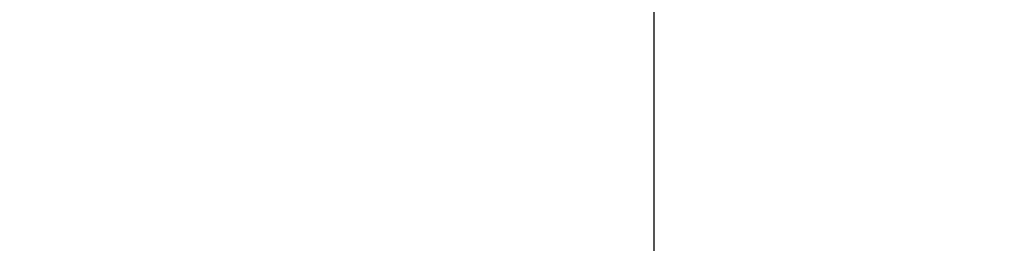
# Model space of a CAD drawing. Units: inches. Extents: x 2083 to 3317, y 1141 to 2115.
# Tile 66 of 256: x 2237.106 to 2238.294, y 1477.926 to 1478.196. Entities that reach past the tile are written whole.
import ezdxf

# ---------------------------------------------------------------- set-up
doc = ezdxf.new("R2010")
doc.units = ezdxf.units.IN
doc.layers.add('A-ANNO-DIMS', color=2, linetype='Continuous', lineweight=18)
doc.layers.add('A-WALL-PATT', color=251, linetype='Continuous', lineweight=13, true_color=0x636466)
doc.styles.get("Standard").update_dxf_attribs({"font": 'arial.ttf'})
doc.dimstyles.new('ISO-25', dxfattribs={"dimtxt": 12, "dimasz": 12, "dimexe": 1.25, "dimexo": 0.625, "dimtad": 1, "dimlunit": 3, "dimtxsty": 'Standard', "dimcen": 2.5, "dimadec": 0, "dimazin": 0, "dimtfac": 1, "dimtmove": 0, "dimatfit": 3, "dimfxl": 1, "dimarcsym": 0})

# ---------------------------------------------------------------- blocks, each defined once
blk = doc.blocks.new('*D30')
at = {"layer": 'A-ANNO-DIMS', "color": 0, "lineweight": -2, "transparency": 16777216}
for p, q in [((2240.0179, 1445.2738), (2240.0179, 1448.0455)), ((2254.3293, 1445.2738), (2254.3293, 1448.0455)), ((2228.0179, 1446.7955), (2216.0179, 1446.7955)), ((2240.0179, 1446.7955), (2254.3293, 1446.7955)), ((2266.3293, 1446.7955), (2413.7649, 1446.7955))]:
    blk.add_line(p, q, dxfattribs=at)
at = {"layer": 'A-ANNO-DIMS', "color": 0, "transparency": 16777216}
for points in [[(2228.0179, 1448.7955), (2228.0179, 1444.7955), (2240.0179, 1446.7955)], [(2266.3293, 1448.7955), (2266.3293, 1444.7955), (2254.3293, 1446.7955)]]:
    blk.add_solid(points, dxfattribs=at)
at = {"layer": 'Defpoints', "color": 0, "transparency": 16777216}
for p in [(2254.3293, 1446.7955), (2240.0179, 1444.6488), (2254.3293, 1444.6488)]:
    blk.add_point(p, dxfattribs=at)
at = {"layer": 'A-ANNO-DIMS', "color": 0, "transparency": 16777216, "insert": (2346.0471, 1453.6252), "char_height": 12, "attachment_point": 5}
blk.add_mtext('WC 1\'-2 1/2" TYP.', dxfattribs=at)
blk = doc.blocks.new('*D31')
at = {"layer": 'A-ANNO-DIMS', "color": 0, "lineweight": -2, "transparency": 16777216}
for p, q in [((2237.8711, 1456.6488), (2237.8711, 1541.9152)), ((2239.3929, 1444.6488), (2236.6211, 1444.6488)), ((2237.8711, 1431.5475), (2237.8711, 1444.6488)), ((2239.3929, 1431.5475), (2236.6211, 1431.5475)), ((2237.8711, 1419.5475), (2237.8711, 1407.5475))]:
    blk.add_line(p, q, dxfattribs=at)
at = {"layer": 'A-ANNO-DIMS', "color": 0, "transparency": 16777216}
for points in [[(2235.8711, 1456.6488), (2239.8711, 1456.6488), (2237.8711, 1444.6488)], [(2235.8711, 1419.5475), (2239.8711, 1419.5475), (2237.8711, 1431.5475)]]:
    blk.add_solid(points, dxfattribs=at)
at = {"layer": 'Defpoints', "color": 0, "transparency": 16777216}
for p in [(2237.8711, 1444.6488), (2240.0179, 1444.6488), (2240.0179, 1431.5475)]:
    blk.add_point(p, dxfattribs=at)
at = {"layer": 'A-ANNO-DIMS', "color": 0, "transparency": 16777216, "insert": (2231.2175, 1505.282), "char_height": 12, "attachment_point": 5, "rotation": 90}
blk.add_mtext('1\'-1" TYP.', dxfattribs=at)
blk = doc.blocks.new('*D45')
at = {"layer": 'A-ANNO-DIMS', "color": 0, "lineweight": -2, "transparency": 16777216}
for p, q in [((2235.9598, 1478.3864), (2235.9598, 1531.3614)), ((2418.9598, 1478.3864), (2418.9598, 1531.3614)), ((2247.9598, 1530.1114), (2406.9598, 1530.1114))]:
    blk.add_line(p, q, dxfattribs=at)
at = {"layer": 'A-ANNO-DIMS', "color": 0, "transparency": 16777216}
for points in [[(2247.9598, 1532.1114), (2247.9598, 1528.1114), (2235.9598, 1530.1114)], [(2406.9598, 1532.1114), (2406.9598, 1528.1114), (2418.9598, 1530.1114)]]:
    blk.add_solid(points, dxfattribs=at)
at = {"layer": 'Defpoints', "color": 0, "transparency": 16777216}
for p in [(2418.9598, 1530.1114), (2235.9598, 1477.7614), (2418.9598, 1477.7614)]:
    blk.add_point(p, dxfattribs=at)
at = {"layer": 'A-ANNO-DIMS', "color": 0, "transparency": 16777216, "insert": (2327.4598, 1536.8673), "char_height": 12, "attachment_point": 5}
blk.add_mtext('15\'-3"', dxfattribs=at)
blk = doc.blocks.new('*D62')
at = {"layer": 'A-ANNO-DIMS', "color": 0, "lineweight": -2, "transparency": 16777216}
for p, q in [((2235.9598, 1469.3864), (2235.9598, 1522.3614)), ((2379.9598, 1469.3864), (2379.9598, 1522.3614)), ((2247.9598, 1521.1114), (2367.9598, 1521.1114))]:
    blk.add_line(p, q, dxfattribs=at)
at = {"layer": 'A-ANNO-DIMS', "color": 0, "transparency": 16777216}
for points in [[(2247.9598, 1523.1114), (2247.9598, 1519.1114), (2235.9598, 1521.1114)], [(2367.9598, 1523.1114), (2367.9598, 1519.1114), (2379.9598, 1521.1114)]]:
    blk.add_solid(points, dxfattribs=at)
at = {"layer": 'Defpoints', "color": 0, "transparency": 16777216}
for p in [(2379.9598, 1521.1114), (2235.9598, 1468.7614), (2379.9598, 1468.7614)]:
    blk.add_point(p, dxfattribs=at)
at = {"layer": 'A-ANNO-DIMS', "color": 0, "transparency": 16777216, "insert": (2307.9598, 1527.8632), "char_height": 12, "attachment_point": 5}
blk.add_mtext('12\'-0"', dxfattribs=at)

msp = doc.modelspace()

# ---------------------------------------------------------------- hatches: boundary and pattern name
at = {"layer": 'A-WALL-PATT'}
h = msp.add_hatch(color=256, dxfattribs=at)
h.dxf.hatch_style = 1
h.paths.add_polyline_path([(3126.9598, 2020.7614), (2748.9598, 2020.7614), (2604.9598, 2020.7614), (2226.9598, 2020.7614), (2226.9598, 1702.7614), (2466.9598, 1702.7614), (2466.9598, 1582.7614), (2418.9598, 1582.7614), (2418.9598, 1477.7614), (2226.9598, 1477.7614), (2226.9598, 1263.2614), (2544.9598, 1263.2614), (2544.9598, 1411.7614), (2604.9598, 1411.7614), (2685.9598, 1411.7614), (2685.9598, 1420.7614), (2604.9598, 1420.7614), (2604.9598, 1573.7614), (2604.9598, 1702.7614), (2604.9598, 2011.7614), (2748.9598, 2011.7614), (2748.9598, 1702.7614), (2862.9598, 1702.7614), (2862.9598, 1621.7614), (2871.9598, 1621.7614), (2871.9598, 1702.7614), (2883.9598, 1702.7614), (2883.9598, 1706.9395, -0.026459), (2883.9598, 1711.7614), (2757.9598, 1711.7614), (2757.9598, 1807.7614), (2787.9598, 1807.7614), (2787.9598, 1812.2614), (2757.9598, 1812.2614), (2757.9598, 2011.7614), (2877.9598, 2011.7614), (2877.9598, 1812.2614), (2847.9598, 1812.2614), (2847.9598, 1807.7614), (2889.8357, 1807.7614), (2889.8357, 1812.2614), (2882.4598, 1812.2614), (2882.4598, 2011.7614), (3117.9598, 2011.7614), (3117.9598, 1812.2614), (2937.8357, 1812.2614), (2937.8357, 1807.7614), (2995.7098, 1807.7614), (2995.7098, 1796.1177), (3000.2098, 1796.1177), (3000.2098, 1807.7614), (3117.9598, 1807.7614), (3117.9598, 1711.7614), (3000.2098, 1711.7614), (3000.2098, 1760.1177), (2998.5727, 1760.1177, -0.020711), (2995.7098, 1760.1177), (2995.7098, 1711.7614), (2931.9598, 1711.7614), (2931.9598, 1702.7614), (3126.9598, 1702.7614)])
h.paths.add_polyline_path([(2471.4598, 2011.7614), (2471.4598, 1810.0114), (2462.7169, 1810.0114), (2462.7169, 1805.5114), (2505.9598, 1805.5114), (2505.9598, 1810.0114), (2475.9598, 1810.0114), (2475.9598, 2011.7614), (2595.9598, 2011.7614), (2595.9598, 1810.0114), (2565.9598, 1810.0114), (2565.9598, 1805.5114), (2595.9598, 1805.5114), (2595.9598, 1711.7614), (2235.9598, 1711.7614), (2235.9598, 1805.5114), (2353.7098, 1805.5114), (2353.7098, 1796.0542), (2358.2098, 1796.0542), (2358.2098, 1805.5114), (2414.7169, 1805.5114), (2414.7169, 1810.0114), (2235.9598, 1810.0114), (2235.9598, 2011.7614)], flags=16)
h.paths.add_polyline_path([(2270.2047, 1994.61), (2270.2047, 1970.61), (2246.2047, 1970.61), (2246.2047, 1994.61)], flags=0)
edge = h.paths.add_edge_path(flags=0)
edge.add_ellipse((2332.0274, 1899.7982), major_axis=(-3.043, 3.043), ratio=0.168252, start_angle=-161.3322, end_angle=-156.3071, ccw=False)
edge.add_ellipse((2333.082, 1898.7435), major_axis=(-1.0546, 1.0546), ratio=0.453532, start_angle=-123.371, end_angle=-94.1591)
edge = h.paths.add_edge_path(flags=0)
edge.add_ellipse((2332.0274, 1968.8763), major_axis=(3.043, 3.043), ratio=0.168252, start_angle=18.6678, end_angle=23.6929)
edge.add_spline(control_points=[(2332.9256, 1970.6911), (2332.2268, 1970.3361), (2330.8937, 1969.6589), (2328.4131, 1970.9321), (2327.2039, 1967.7487), (2324.7096, 1969.9556), (2322.5328, 1967.0124), (2320.0128, 1971.2958), (2317.6803, 1968.1578), (2316.0405, 1967.102), (2315.4269, 1966.8096)], knot_values=[0, 0, 0, 0, 2.267059, 4.324559, 6.685584, 8.878641, 11.121502, 14.300359, 17.755284, 19.732645, 19.732645, 19.732645, 19.732645], degree=3, periodic=0)
edge.add_ellipse((2332.0274, 1968.8763), major_axis=(3.043, 3.043), ratio=0.168252, start_angle=18.6678, end_angle=23.6929, ccw=False)
edge.add_ellipse((2333.082, 1969.9309), major_axis=(1.0546, 1.0546), ratio=0.453532, start_angle=56.629, end_angle=85.8409, ccw=False)
edge = h.paths.add_edge_path(flags=0)
edge.add_spline(control_points=[(2296.4283, 1967.9879), (2293.6278, 1965.3363), (2287.7036, 1959.7271), (2299.7439, 1949.9957), (2294.5326, 1935.6685), (2290.5732, 1920.6035), (2293.3941, 1909.9737), (2296.1854, 1904.9665)], knot_values=[0.099185, 0.099185, 0.099185, 0.099185, 0.345301, 0.619822, 0.982653, 1.386093, 1.810555, 1.810555, 1.810555, 1.810555], degree=3, periodic=0)
edge.add_spline(control_points=[(2296.1854, 1904.9665), (2297.3836, 1902.6193), (2298.001, 1901.9493), (2298.553, 1901.4682)], knot_values=[0.006246, 0.006246, 0.006246, 0.006246, 0.055476, 0.055476, 0.055476, 0.055476], degree=3, periodic=0)
edge.add_spline(control_points=[(2298.553, 1901.4682), (2297.2586, 1900.9232), (2295.2253, 1900.2321), (2293.0602, 1900.6142), (2292.1014, 1900.7884), (2292.0896, 1900.7906)], knot_values=[0.312835, 0.312835, 0.312835, 0.312835, 0.40178, 0.474987, 0.475903, 0.475903, 0.475903, 0.475903], degree=3, periodic=0)
edge.add_arc((2292.7936, 1904.6641), 3.937, 215.4209, 259.6982, ccw=False)
edge.add_spline(control_points=[(2289.5853, 1902.3823), (2289.4767, 1902.5351), (2289.3685, 1902.688), (2289.2609, 1902.8412)], knot_values=[0.102872, 0.102872, 0.102872, 0.102872, 0.116896, 0.116896, 0.116896, 0.116896], degree=3, periodic=0)
edge.add_spline(control_points=[(2289.2609, 1902.8412), (2288.6866, 1902.5502), (2287.64, 1902.0199), (2285.8813, 1901.874), (2283.853, 1901.5044), (2281.72, 1899.7105), (2278.467, 1899.4929), (2276.1571, 1901.8832), (2272.259, 1899.8041), (2267.7776, 1901.8432), (2262.2439, 1900.184), (2257.4149, 1901.7821), (2254.3184, 1900.7261), (2253.1783, 1900.3373)], knot_values=[0, 0, 0, 0, 1.907977, 3.477176, 5.261074, 7.972851, 11.680248, 13.717921, 16.939592, 22.789562, 27.502503, 33.595215, 37.145618, 37.145618, 37.145618, 37.145618], degree=3, periodic=0)
edge.add_line((2253.1783, 1900.3373), (2250.2442, 1902.8412))
edge.add_line((2250.2442, 1902.8412), (2250.2442, 1965.8333))
edge.add_line((2250.2442, 1965.8333), (2253.1783, 1968.3371))
edge.add_spline(control_points=[(2253.1783, 1968.3371), (2254.3184, 1967.9483), (2257.4149, 1966.8924), (2262.2439, 1968.4904), (2267.7776, 1966.8313), (2271.5267, 1968.5372), (2273.8759, 1967.8283), (2274.2067, 1967.7276)], knot_values=[0, 0, 0, 0, 0.09018, 0.244935, 0.364644, 0.513233, 0.537855, 0.537855, 0.537855, 0.537855], degree=3, periodic=0)
edge.add_arc((2274.3529, 1963.7933), 3.937, 72.0511, 92.1279, ccw=False)
edge.add_arc((2281.2969, 1985.23), 18.5963, 252.05113, 288.56572)
edge.add_arc((2292.3167, 1956.0289), 12.6461, 71.02679, 113.77822, ccw=False)
edge = h.paths.add_edge_path(flags=0)
edge.add_spline(control_points=[(2274.8994, 1951.8562), (2275.0662, 1951.6166), (2275.2327, 1951.3766), (2275.398, 1951.1359)], knot_values=[1.409916, 1.409916, 1.409916, 1.409916, 1.43159, 1.43159, 1.43159, 1.43159], degree=3, periodic=0)
edge.add_spline(control_points=[(2275.398, 1951.1359), (2275.7921, 1950.5619), (2276.1792, 1949.9838), (2276.5455, 1949.3971)], knot_values=[1.358238, 1.358238, 1.358238, 1.358238, 1.409916, 1.409916, 1.409916, 1.409916], degree=3, periodic=0)
edge.add_line((2276.5455, 1949.3971), (2277.4373, 1947.8622))
edge.add_spline(control_points=[(2277.4373, 1947.8622), (2276.3038, 1945.6731), (2274.6397, 1942.4269), (2274.6316, 1938.0939), (2272.7991, 1930.8515), (2274.3564, 1943.897), (2275.9477, 1947.9234), (2276.5455, 1949.3971)], knot_values=[0.005632, 0.005632, 0.005632, 0.005632, 0.186014, 0.266002, 0.357087, 0.59639, 0.739732, 0.739732, 0.739732, 0.739732], degree=3, periodic=0)
edge.add_spline(control_points=[(2276.5455, 1949.3971), (2276.1792, 1949.9838), (2275.7921, 1950.5619), (2275.398, 1951.1359)], knot_values=[1.358238, 1.358238, 1.358238, 1.358238, 1.409916, 1.409916, 1.409916, 1.409916], degree=3, periodic=0)
edge.add_spline(control_points=[(2275.398, 1951.1359), (2274.9425, 1950.0805), (2274.2078, 1948.0253), (2273.9346, 1944.8515), (2272.4685, 1937.6275), (2273.4662, 1945.6965), (2274.7006, 1951.0595), (2274.8994, 1951.8562)], knot_values=[0.104364, 0.104364, 0.104364, 0.104364, 0.189636, 0.269624, 0.36071, 0.600013, 0.644622, 0.644622, 0.644622, 0.644622], degree=3, periodic=0)
h.paths.add_polyline_path([(2269.1675, 1963.1276, -0.357527), (2268.1706, 1960.9764, -0.092561), (2268.1706, 1939.4363, -0.357527), (2269.1675, 1937.2851, -0.357527), (2267.0163, 1938.282, -0.164785), (2254.6856, 1938.282, -0.357527), (2252.5344, 1937.2851, -0.357527), (2253.5313, 1939.4363, -0.092561), (2253.5313, 1960.9764, -0.357527), (2252.5344, 1963.1276, -0.357527), (2254.6856, 1962.1307, -0.164785), (2267.0163, 1962.1307, -0.357527)], flags=0)
h.paths.add_polyline_path([(2248.8741, 1967.8018), (2248.8741, 1957.0277), (2249.4578, 1957.0277), (2249.4578, 1911.6468), (2248.8741, 1911.6468), (2248.8741, 1900.8727), (2246.5119, 1900.8727, 0.197327), (2244.1497, 1902.4569), (2244.1497, 1966.2176, 0.197327), (2246.5119, 1967.8018)], flags=0)
h.paths.add_polyline_path([(2269.1675, 1931.3893, -0.357527), (2268.1706, 1929.2381, -0.092561), (2268.1706, 1907.6981, -0.357527), (2269.1675, 1905.5469, -0.357527), (2267.0163, 1906.5438, -0.164785), (2254.6856, 1906.5438, -0.357527), (2252.5344, 1905.5469, -0.357527), (2253.5313, 1907.6981, -0.092561), (2253.5313, 1929.2381, -0.357527), (2252.5344, 1931.3893, -0.357527), (2254.6856, 1930.3925, -0.164785), (2267.0163, 1930.3925, -0.357527)], flags=0)
edge = h.paths.add_edge_path(flags=0)
edge.add_spline(control_points=[(2276.1969, 1906.7237), (2276.1681, 1909.0289), (2276.114, 1913.3719), (2270.5984, 1924.925), (2273.9052, 1919.0128), (2275.9217, 1916.2621), (2275.4746, 1912.4021), (2277.2579, 1910.3806), (2276.696, 1908.225), (2276.6462, 1906.813), (2276.6178, 1906.0084)], knot_values=[0, 0, 0, 0, 8.61026, 16.221274, 18.843057, 23.804898, 27.440828, 29.356102, 31.203478, 33.650687, 33.650687, 33.650687, 33.650687], degree=3, periodic=0)
edge.add_spline(control_points=[(2276.6178, 1906.0084), (2276.6233, 1905.6241), (2276.4977, 1904.6287), (2275.4418, 1903.8547), (2274.9373, 1903.0804), (2274.8591, 1902.8412)], knot_values=[0.156488, 0.156488, 0.156488, 0.156488, 0.184398, 0.231376, 0.250598, 0.250598, 0.250598, 0.250598], degree=3, periodic=0)
edge.add_line((2274.8591, 1902.8412), (2276.506, 1902.8412))
edge.add_spline(control_points=[(2276.506, 1902.8412), (2276.7883, 1903.0849), (2277.6651, 1904.1252), (2278.2495, 1904.3407), (2277.6539, 1908.5274), (2278.1557, 1906.2278), (2278.1005, 1905.2859), (2278.8467, 1904.069), (2277.8568, 1903.4149), (2277.8742, 1902.991), (2277.9036, 1902.8412)], knot_values=[0.059574, 0.059574, 0.059574, 0.059574, 0.080753, 0.103741, 0.16972, 0.176036, 0.207137, 0.240474, 0.262341, 0.27366, 0.27366, 0.27366, 0.27366], degree=3, periodic=0)
edge.add_line((2277.9036, 1902.8412), (2280.0298, 1902.8412))
edge.add_spline(control_points=[(2280.0298, 1902.8412), (2279.8882, 1903.0884), (2279.4993, 1903.9816), (2280.1523, 1905.9393), (2278.1036, 1909.6578), (2279.7624, 1907.1853), (2280.3279, 1904.8749), (2280.4851, 1903.4896), (2281.4633, 1903.2494), (2281.7583, 1902.9365), (2281.834, 1902.8412)], knot_values=[0.013856, 0.013856, 0.013856, 0.013856, 0.034874, 0.088867, 0.107879, 0.126738, 0.158714, 0.193757, 0.217487, 0.226722, 0.226722, 0.226722, 0.226722], degree=3, periodic=0)
edge.add_spline(control_points=[(2281.834, 1902.8412), (2281.7875, 1902.8267), (2281.647, 1902.783), (2281.3955, 1902.8595), (2281.0881, 1902.9852), (2280.7207, 1903.0609), (2280.3335, 1903.0257), (2280.1248, 1902.8989), (2280.0298, 1902.8412)], knot_values=[0, 0, 0, 0, 0.14413, 0.435517, 0.749276, 1.153046, 1.548371, 1.878348, 1.878348, 1.878348, 1.878348], degree=3, periodic=0)
edge.add_line((2280.0298, 1902.8412), (2277.9036, 1902.8412))
edge.add_spline(control_points=[(2277.9036, 1902.8412), (2277.8929, 1902.7959), (2277.8654, 1902.6796), (2277.6075, 1902.6875), (2277.2741, 1902.8007), (2276.8379, 1902.6198), (2276.5838, 1902.7893), (2276.506, 1902.8412)], knot_values=[0, 0, 0, 0, 0.127189, 0.326199, 0.628009, 1.24357, 1.515331, 1.515331, 1.515331, 1.515331], degree=3, periodic=0)
edge.add_line((2276.506, 1902.8412), (2274.8591, 1902.8412))
edge.add_spline(control_points=[(2274.8591, 1902.8412), (2274.8144, 1902.8986), (2274.7251, 1903.0134), (2274.4935, 1903.119), (2274.2443, 1902.9605), (2273.9371, 1903.1849), (2273.614, 1902.9831), (2273.4083, 1902.883), (2273.3223, 1902.8412)], knot_values=[0, 0, 0, 0, 0.21843, 0.436957, 0.687977, 0.990379, 1.398396, 1.69185, 1.69185, 1.69185, 1.69185], degree=3, periodic=0)
edge.add_spline(control_points=[(2273.3223, 1902.8412), (2273.6167, 1903.4457), (2274.274, 1904.5383), (2276.0272, 1904.5737), (2276.207, 1906.5836), (2276.1969, 1906.7237)], knot_values=[0.012227, 0.012227, 0.012227, 0.012227, 0.059472, 0.106218, 0.134458, 0.134458, 0.134458, 0.134458], degree=3, periodic=0)
h.paths.add_polyline_path([(2270.7761, 1897.7898), (2270.7761, 1873.7898), (2246.7761, 1873.7898), (2246.7761, 1897.7898)], flags=0)
h.paths.add_polyline_path([(2353.7098, 1760.0051), (2353.7098, 1760.0542), (2358.2098, 1760.0542, -0.033729)], flags=0)
h.paths.add_polyline_path([(2321.8191, 1737.5292), (2341.9953, 1737.5292, -0.414214), (2343.2033, 1736.3212), (2343.2033, 1721.0206, -0.414214), (2341.9953, 1719.8127), (2321.8191, 1719.8127, -0.414214), (2320.6112, 1721.0206), (2320.6112, 1736.3212, -0.414214)], flags=0)
h.paths.add_polyline_path([(2324.235, 1736.3212), (2339.5794, 1736.3212, -0.414214), (2341.9953, 1733.9053), (2341.9953, 1725.4497, -0.414214), (2339.5794, 1723.0338), (2333.6806, 1723.0338), (2333.8453, 1722.0455, -0.870646), (2335.4254, 1721.8259, -0.767327), (2333.9227, 1721.4232), (2331.291, 1721.4232, -0.767327), (2329.7883, 1721.8259, -0.870646), (2331.3684, 1722.0455), (2331.5331, 1723.0338), (2324.235, 1723.0338, -0.414214), (2321.8191, 1725.4497), (2321.8191, 1733.9053, -0.414214)], flags=0)
h.paths.add_polyline_path([(2570.4838, 1928.6154), (2589.6838, 1928.6154), (2590.1688, 1928.6154), (2590.1688, 1904.9934), (2570.4838, 1904.9934)], flags=0)
h.paths.add_polyline_path([(2574.4473, 1927.2638, -1), (2572.8288, 1927.2638, -1)], flags=0)
h.paths.add_polyline_path([(2573.0899, 1926.9409), (2573.925, 1927.776), (2574.1477, 1927.5533), (2573.3126, 1926.7182)], flags=0)
h.paths.add_polyline_path([(2578.7791, 1919.7296, -1), (2571.5917, 1919.7296, -1)], flags=0)
h.paths.add_polyline_path([(2578.3854, 1919.7296, -1), (2571.9854, 1919.7296, -1)], flags=0)
h.paths.add_polyline_path([(2331.5958, 1729.4762, -1), (2333.618, 1729.4762, -1)], flags=0)
h.paths.add_polyline_path([(2578.0342, 1927.2638, -1), (2576.4157, 1927.2638, -1)], flags=0)
h.paths.add_polyline_path([(2576.6889, 1927.5311), (2576.9116, 1927.7538), (2577.7467, 1926.9186), (2577.524, 1926.6959)], flags=0)
h.paths.add_polyline_path([(2578.1391, 1909.8595, -1), (2572.2317, 1909.8595, -1)], flags=0)
h.paths.add_polyline_path([(2577.7454, 1909.8595, -1), (2572.6254, 1909.8595, -1)], flags=0)
h.paths.add_polyline_path([(2583.7977, 1927.2638, -1), (2582.1792, 1927.2638, -1)], flags=0)
h.paths.add_polyline_path([(2582.7186, 1927.7538), (2583.5538, 1926.9186), (2583.3311, 1926.6959), (2582.4959, 1927.5311)], flags=0)
h.paths.add_polyline_path([(2582.4959, 1927.5311), (2582.7186, 1927.7538), (2583.5538, 1926.9186), (2583.3311, 1926.6959)], flags=0)
h.paths.add_polyline_path([(2587.7391, 1920.5296, -1), (2581.8317, 1920.5296, -1)], flags=0)
h.paths.add_polyline_path([(2587.3454, 1920.5296, -1), (2582.2254, 1920.5296, -1)], flags=0)
h.paths.add_polyline_path([(2587.3846, 1927.2638, -1), (2585.7661, 1927.2638, -1)], flags=0)
h.paths.add_polyline_path([(2586.082, 1926.9802), (2586.9172, 1927.8154), (2587.1399, 1927.5927), (2586.3047, 1926.7575)], flags=0)
h.paths.add_polyline_path([(2588.3791, 1910.6595, -1), (2581.1917, 1910.6595, -1)], flags=0)
h.paths.add_polyline_path([(2587.9854, 1910.6595, -1), (2581.5854, 1910.6595, -1)], flags=0)
h.paths.add_polyline_path([(2417.1677, 1729.4779), (2437.3439, 1729.4779, -0.414214), (2438.5519, 1728.2699), (2438.5519, 1712.9693, -0.414214), (2437.3439, 1711.7614), (2417.1677, 1711.7614, -0.414214), (2415.9598, 1712.9693), (2415.9598, 1728.2699, -0.414214)], flags=0)
h.paths.add_polyline_path([(2419.5836, 1728.2699), (2434.928, 1728.2699, -0.414214), (2437.3439, 1725.8541), (2437.3439, 1717.3984, -0.414214), (2434.928, 1714.9825), (2429.0292, 1714.9825), (2429.1939, 1713.9942, -0.870646), (2430.774, 1713.7746, -0.767327), (2429.2713, 1713.372), (2426.6396, 1713.372, -0.767327), (2425.1369, 1713.7746, -0.870646), (2426.717, 1713.9942), (2426.8817, 1714.9825), (2419.5836, 1714.9825, -0.414214), (2417.1677, 1717.3984), (2417.1677, 1725.8541, -0.414214)], flags=0)
h.paths.add_polyline_path([(2419.5836, 1728.2699), (2434.928, 1728.2699, -0.414214), (2437.3439, 1725.8541), (2437.3439, 1717.3984, -0.414214), (2434.928, 1714.9825), (2429.0292, 1714.9825), (2428.3581, 1719.009), (2427.5528, 1719.009), (2426.8817, 1714.9825), (2419.5836, 1714.9825, -0.414214), (2417.1677, 1717.3984), (2417.1677, 1725.8541, -0.414214)], flags=0)
h.paths.add_polyline_path([(2426.9444, 1721.4249, -1), (2428.9666, 1721.4249, -1)], flags=0)
h.paths.add_polyline_path([(2475.9598, 1702.7614), (2595.9598, 1702.7614), (2595.9598, 1582.7614), (2475.9598, 1582.7614)], flags=16)
h.paths.add_polyline_path([(2427.9598, 1573.7614), (2595.9598, 1573.7614), (2595.9598, 1468.7614), (2595.9598, 1420.7614), (2384.4598, 1420.7614), (2384.4598, 1468.7614), (2427.9598, 1468.7614)], flags=16)
h.paths.add_polyline_path([(2379.9598, 1468.7614), (2379.9598, 1420.7614), (2235.9598, 1420.7614), (2235.9598, 1468.7614)], flags=16)
h.paths.add_polyline_path([(2317.816, 1466.6958), (2337.9922, 1466.6958, -0.414214), (2339.2002, 1465.4878), (2339.2002, 1450.1872, -0.414214), (2337.9922, 1448.9792), (2317.816, 1448.9792, -0.414214), (2316.6081, 1450.1872), (2316.6081, 1465.4878, -0.414214)], flags=0)
h.paths.add_polyline_path([(2320.2319, 1465.4878), (2335.5763, 1465.4878, -0.414214), (2337.9922, 1463.0719), (2337.9922, 1454.6163, -0.414214), (2335.5763, 1452.2004), (2329.6775, 1452.2004), (2329.8422, 1451.212, -0.870646), (2331.4223, 1450.9925, -0.767327), (2329.9196, 1450.5898), (2327.2879, 1450.5898, -0.767327), (2325.7852, 1450.9925, -0.870646), (2327.3653, 1451.212), (2327.53, 1452.2004), (2320.2319, 1452.2004, -0.414214), (2317.816, 1454.6163), (2317.816, 1463.0719, -0.414214)], flags=0)
h.paths.add_polyline_path([(2320.2319, 1465.4878), (2335.5763, 1465.4878, -0.414214), (2337.9922, 1463.0719), (2337.9922, 1454.6163, -0.414214), (2335.5763, 1452.2004), (2329.6775, 1452.2004), (2329.0064, 1456.2269), (2328.2011, 1456.2269), (2327.53, 1452.2004), (2320.2319, 1452.2004, -0.414214), (2317.816, 1454.6163), (2317.816, 1463.0719, -0.414214)], flags=0)
h.paths.add_polyline_path([(2327.5926, 1458.6428, -1), (2329.6148, 1458.6428, -1)], flags=0)
h.paths.add_polyline_path([(2244.4117, 1433.3405), (2241.9209, 1433.3405, -0.414214), (2240.0179, 1435.2435), (2240.0179, 1440.9528, -0.414211), (2241.9209, 1442.8559), (2244.4117, 1442.8559, -1.976472)], flags=0)
h.paths.add_polyline_path([(2245.3569, 1434.3975, -0.414214), (2245.3569, 1441.7988, -2.144098)], flags=0)
h.paths.add_polyline_path([(2535.9598, 1416.2614), (2535.9598, 1272.2614), (2235.9598, 1272.2614), (2235.9598, 1416.2614)], flags=16)
h.paths.add_polyline_path([(2260.1196, 1384.2928), (2260.1196, 1362.0386), (2237.8654, 1362.0386), (2237.8654, 1384.2928)], flags=0)
edge = h.paths.add_edge_path(flags=0)
edge.add_line((2318.2518, 1362.0933), (2318.1458, 1362.001))
edge.add_ellipse((2317.4451, 1360.431), major_axis=(2.8216, 2.8216), ratio=0.168252, start_angle=18.6678, end_angle=20.9481, ccw=False)
edge.add_ellipse((2318.423, 1361.409), major_axis=(0.9779, 0.9779), ratio=0.453532, start_angle=56.629, end_angle=70.2262, ccw=False)
edge = h.paths.add_edge_path(flags=0)
edge.add_line((2319.1074, 1295.5711), (2319.015, 1295.6771))
edge.add_ellipse((2317.4451, 1296.3778), major_axis=(-2.8216, 2.8216), ratio=0.168252, start_angle=-161.3322, end_angle=-159.0519, ccw=False)
edge.add_ellipse((2318.423, 1295.3999), major_axis=(-0.9779, 0.9779), ratio=0.453532, start_angle=-123.371, end_angle=-109.7738)
edge = h.paths.add_edge_path(flags=0)
edge.add_spline(control_points=[(2284.2103, 1301.1702), (2284.5807, 1300.4447), (2284.8912, 1299.892), (2285.1596, 1299.461)], knot_values=[0.039066, 0.039066, 0.039066, 0.039066, 0.055476, 0.055476, 0.055476, 0.055476], degree=3, periodic=0)
edge.add_line((2285.1596, 1299.461), (2284.2103, 1301.1702))
edge = h.paths.add_edge_path(flags=0)
edge.add_line((2280.4125, 1297.298), (2283.37, 1297.0361))
edge.add_line((2283.37, 1297.0361), (2286.4057, 1297.9263))
edge.add_spline(control_points=[(2286.4057, 1297.9263), (2285.3055, 1297.4631), (2284.3448, 1297.1292), (2283.37, 1297.0361)], knot_values=[0.394369, 0.394369, 0.394369, 0.394369, 0.475903, 0.475903, 0.475903, 0.475903], degree=3, periodic=0)
edge.add_spline(control_points=[(2283.37, 1297.0361), (2283.2814, 1297.0277), (2282.3163, 1296.9573), (2281.3125, 1297.1345), (2280.4234, 1297.296), (2280.4125, 1297.298)], knot_values=[0.312835, 0.312835, 0.312835, 0.312835, 0.320246, 0.393453, 0.394369, 0.394369, 0.394369, 0.394369], degree=3, periodic=0)
edge = h.paths.add_edge_path(flags=0)
edge.add_line((2284.4356, 1359.6073), (2280.4463, 1355.328))
edge.add_line((2280.4463, 1355.328), (2279.58, 1351.0178))
edge.add_line((2279.58, 1351.0178), (2282.413, 1346.5804))
edge.add_spline(control_points=[(2282.413, 1346.5804), (2283.1533, 1345.5892), (2284.2529, 1344.0289), (2284.801, 1342.3872), (2284.9352, 1341.8055)], knot_values=[1.240098, 1.240098, 1.240098, 1.240098, 1.332892, 1.382712, 1.382712, 1.382712, 1.382712], degree=3, periodic=0)
edge.add_spline(control_points=[(2284.9352, 1341.8055), (2285.3191, 1340.1406), (2285.233, 1338.4092), (2284.9099, 1336.6541)], knot_values=[1.097484, 1.097484, 1.097484, 1.097484, 1.240098, 1.240098, 1.240098, 1.240098], degree=3, periodic=0)
edge.add_spline(control_points=[(2284.9099, 1336.6541), (2284.5868, 1334.899), (2284.0267, 1333.1203), (2283.4626, 1331.3606)], knot_values=[0.95487, 0.95487, 0.95487, 0.95487, 1.097484, 1.097484, 1.097484, 1.097484], degree=3, periodic=0)
edge.add_line((2283.4626, 1331.3606), (2281.8904, 1326.1534))
edge.add_line((2281.8904, 1326.1534), (2280.7563, 1321.0561))
edge.add_line((2280.7563, 1321.0561), (2280.2992, 1316.002))
edge.add_line((2280.2992, 1316.002), (2280.7159, 1310.9501))
edge.add_line((2280.7159, 1310.9501), (2282.0281, 1305.9721))
edge.add_line((2282.0281, 1305.9721), (2284.2103, 1301.1702))
edge.add_spline(control_points=[(2284.2103, 1301.1702), (2283.3407, 1302.7302), (2282.6119, 1304.3365), (2282.0281, 1305.9721)], knot_values=[0.099185, 0.099185, 0.099185, 0.099185, 0.241799, 0.241799, 0.241799, 0.241799], degree=3, periodic=0)
edge.add_spline(control_points=[(2282.0281, 1305.9721), (2281.4443, 1307.6078), (2281.0055, 1309.2728), (2280.7159, 1310.9501)], knot_values=[0.241799, 0.241799, 0.241799, 0.241799, 0.384413, 0.384413, 0.384413, 0.384413], degree=3, periodic=0)
edge.add_spline(control_points=[(2280.7159, 1310.9501), (2280.4332, 1312.5876), (2280.2894, 1314.277), (2280.2989, 1315.962), (2280.2992, 1316.002)], knot_values=[0.384413, 0.384413, 0.384413, 0.384413, 0.523647, 0.527028, 0.527028, 0.527028, 0.527028], degree=3, periodic=0)
edge.add_spline(control_points=[(2280.2992, 1316.002), (2280.3123, 1317.687), (2280.4779, 1319.3679), (2280.7563, 1321.0561)], knot_values=[0.527028, 0.527028, 0.527028, 0.527028, 0.669642, 0.669642, 0.669642, 0.669642], degree=3, periodic=0)
edge.add_spline(control_points=[(2280.7563, 1321.0561), (2281.0346, 1322.7443), (2281.4259, 1324.4396), (2281.8904, 1326.1534)], knot_values=[0.669642, 0.669642, 0.669642, 0.669642, 0.812256, 0.812256, 0.812256, 0.812256], degree=3, periodic=0)
edge.add_spline(control_points=[(2281.8904, 1326.1534), (2282.2644, 1327.5333), (2282.7879, 1329.2618), (2283.3528, 1331.0178), (2283.4626, 1331.3606)], knot_values=[0.812256, 0.812256, 0.812256, 0.812256, 0.927087, 0.95487, 0.95487, 0.95487, 0.95487], degree=3, periodic=0)
edge.add_line((2283.4626, 1331.3606), (2284.9099, 1336.6541))
edge.add_line((2284.9099, 1336.6541), (2284.9352, 1341.8055))
edge.add_line((2284.9352, 1341.8055), (2282.413, 1346.5804))
edge.add_spline(control_points=[(2282.413, 1346.5804), (2281.2751, 1348.1038), (2280.0784, 1349.5703), (2279.58, 1351.0178)], knot_values=[1.382712, 1.382712, 1.382712, 1.382712, 1.525326, 1.525326, 1.525326, 1.525326], degree=3, periodic=0)
edge.add_spline(control_points=[(2279.58, 1351.0178), (2279.4433, 1351.4147), (2279.1363, 1352.8569), (2279.7352, 1354.2904), (2280.4463, 1355.328)], knot_values=[1.525326, 1.525326, 1.525326, 1.525326, 1.564439, 1.667941, 1.667941, 1.667941, 1.667941], degree=3, periodic=0)
edge.add_spline(control_points=[(2280.4463, 1355.328), (2281.4261, 1356.7578), (2282.9308, 1358.1826), (2284.4356, 1359.6073)], knot_values=[1.667941, 1.667941, 1.667941, 1.667941, 1.810555, 1.810555, 1.810555, 1.810555], degree=3, periodic=0)
edge.add_arc((2280.6231, 1348.5182), 11.7262, 71.02679, 113.77822)
edge.add_arc((2270.4049, 1375.5952), 17.2436, 252.05113, 288.56572, ccw=False)
edge.add_arc((2263.966, 1355.7178), 3.6506, 72.0511, 92.1279)
edge.add_arc((2263.966, 1355.7178), 3.6506, 92.1279, 177.9851)
edge.add_spline(control_points=[(2260.3176, 1355.8462), (2260.2604, 1354.2207), (2260.5513, 1350.1865), (2262.9993, 1346.7663), (2264.4727, 1344.649)], knot_values=[1.43159, 1.43159, 1.43159, 1.43159, 1.564144, 1.770695, 1.770695, 1.770695, 1.770695], degree=3, periodic=0)
edge.add_line((2264.4727, 1344.649), (2264.9356, 1343.9825))
edge.add_spline(control_points=[(2263.801, 1340.2481), (2263.8432, 1340.5141), (2264.0672, 1341.7565), (2264.5127, 1343.0025), (2264.935, 1343.9811)], knot_values=[0.53657, 0.53657, 0.53657, 0.53657, 0.559349, 0.644622, 0.644622, 0.644622, 0.644622], degree=3, periodic=0)
edge.add_spline(control_points=[(2264.935, 1343.9811), (2265.1178, 1343.715), (2265.2989, 1343.4479), (2265.4768, 1343.1794)], knot_values=[1.384077, 1.384077, 1.384077, 1.384077, 1.409916, 1.409916, 1.409916, 1.409916], degree=3, periodic=0)
edge.add_spline(control_points=[(2265.4768, 1343.1794), (2265.6546, 1342.9108), (2265.8293, 1342.6408), (2265.9991, 1342.3688)], knot_values=[1.358238, 1.358238, 1.358238, 1.358238, 1.384077, 1.384077, 1.384077, 1.384077], degree=3, periodic=0)
edge.add_line((2265.9991, 1342.3688), (2266.826, 1340.9455))
edge.add_spline(control_points=[(2266.826, 1340.9455), (2268.8944, 1337.0897), (2271.3982, 1325.843), (2270.5162, 1310.5686), (2275.9194, 1301.8606), (2277.7895, 1299.1994)], knot_values=[0.116896, 0.116896, 0.116896, 0.116896, 0.472987, 1.050969, 1.313793, 1.313793, 1.313793, 1.313793], degree=3, periodic=0)
edge.add_spline(control_points=[(2277.7895, 1299.1994), (2277.8394, 1299.1285), (2277.8894, 1299.0575), (2277.9396, 1298.9866)], knot_values=[0.109884, 0.109884, 0.109884, 0.109884, 0.116896, 0.116896, 0.116896, 0.116896], degree=3, periodic=0)
edge.add_line((2277.9396, 1298.9866), (2277.7888, 1299.1991))
edge.add_spline(control_points=[(2277.7888, 1299.1991), (2277.2566, 1298.9294), (2276.2864, 1298.4379), (2275.0394, 1298.3344), (2274.3833, 1298.2389), (2274.2153, 1298.2093)], knot_values=[33.12187, 33.12187, 33.12187, 33.12187, 35.029056, 36.598255, 37.144827, 37.144827, 37.144827, 37.144827], degree=3, periodic=0)
edge.add_line((2274.2153, 1298.2093), (2273.0731, 1297.893))
edge.add_spline(control_points=[(2273.0731, 1297.893), (2272.3229, 1297.5798), (2271.0392, 1296.5105), (2269.2484, 1296.2261), (2268.4231, 1296.3747)], knot_values=[26.532584, 26.532584, 26.532584, 26.532584, 29.198919, 31.839101, 31.839101, 31.839101, 31.839101], degree=3, periodic=0)
edge.add_line((2268.4231, 1296.3747), (2263.8785, 1297.4575))
edge.add_spline(control_points=[(2263.8785, 1297.4575), (2263.5561, 1297.3594), (2261.8603, 1296.8387), (2260.2388, 1297.2824), (2258.9335, 1297.5165)], knot_values=[15.919551, 15.919551, 15.919551, 15.919551, 16.939592, 21.226067, 21.226067, 21.226067, 21.226067], degree=3, periodic=0)
edge.add_line((2258.9335, 1297.5165), (2254.0552, 1297.329))
edge.add_spline(control_points=[(2254.0552, 1297.329), (2253.7555, 1297.2958), (2252.1137, 1297.1652), (2250.4619, 1297.5442), (2249.1297, 1297.6679)], knot_values=[5.306517, 5.306517, 5.306517, 5.306517, 6.276435, 10.613034, 10.613034, 10.613034, 10.613034], degree=3, periodic=0)
edge.add_line((2249.1297, 1297.6679), (2244.3316, 1296.8778))
edge.add_line((2244.3316, 1296.8778), (2241.611, 1299.1994))
edge.add_line((2241.611, 1299.1994), (2241.611, 1357.6094))
edge.add_line((2241.611, 1357.6094), (2244.3316, 1359.9311))
edge.add_line((2244.3316, 1359.9311), (2252.7288, 1359.5427))
edge.add_spline(control_points=[(2252.7288, 1359.5427), (2252.8709, 1359.5464), (2253.3057, 1359.5482), (2253.7398, 1359.5143), (2254.0317, 1359.4824)], knot_values=[0.233291, 0.233291, 0.233291, 0.233291, 0.244935, 0.268927, 0.268927, 0.268927, 0.268927], degree=3, periodic=0)
edge.add_line((2254.0317, 1359.4824), (2259.5872, 1359.4164))
edge.add_spline(control_points=[(2259.5872, 1359.4164), (2260.6771, 1359.6285), (2262.0732, 1359.897), (2263.5237, 1359.4593), (2263.8304, 1359.366)], knot_values=[0.422516, 0.422516, 0.422516, 0.422516, 0.513233, 0.537855, 0.537855, 0.537855, 0.537855], degree=3, periodic=0)
edge.add_arc((2263.966, 1355.7178), 3.6506, 72.0511, 92.1279, ccw=False)
edge.add_arc((2270.4049, 1375.5952), 17.2436, 252.05113, 288.56572)
edge.add_arc((2280.6231, 1348.5182), 11.7262, 71.02679, 113.77822, ccw=False)
h.paths.add_polyline_path([(2240.3405, 1359.4347), (2240.3405, 1349.4444), (2240.8818, 1349.4444), (2240.8818, 1307.3645), (2240.3405, 1307.3645), (2240.3405, 1297.3741), (2238.1502, 1297.3741, 0.197327), (2235.9598, 1298.8431), (2235.9598, 1357.9657, 0.197327), (2238.1502, 1359.4347)], flags=0)
h.paths.add_polyline_path([(2259.1578, 1355.1005, -0.357527), (2258.2334, 1353.1058, -0.092561), (2258.2334, 1333.1326, -0.357527), (2259.1578, 1331.1379, -0.357527), (2257.1631, 1332.0622, -0.164785), (2245.7293, 1332.0622, -0.357527), (2243.7346, 1331.1379, -0.357527), (2244.6589, 1333.1326, -0.092561), (2244.6589, 1353.1058, -0.357527), (2243.7346, 1355.1005, -0.357527), (2245.7293, 1354.1761, -0.164785), (2257.1631, 1354.1761, -0.357527)], flags=0)
edge = h.paths.add_edge_path(flags=0)
edge.add_line((2265.9991, 1342.3688), (2266.826, 1340.9455))
edge.add_line((2266.826, 1340.9455), (2265.3076, 1337.8141))
edge.add_line((2265.3076, 1337.8141), (2264.3582, 1334.6529))
edge.add_line((2264.3582, 1334.6529), (2264.262, 1333.7997))
edge.add_spline(control_points=[(2264.262, 1333.7997), (2264.2084, 1333.1871), (2264.1621, 1332.3655), (2264.0071, 1331.4139), (2263.969, 1331.2018)], knot_values=[0.464444, 0.464444, 0.464444, 0.464444, 0.516691, 0.531608, 0.531608, 0.531608, 0.531608], degree=3, periodic=0)
edge.add_spline(control_points=[(2263.969, 1331.2018), (2263.7745, 1330.1189), (2263.4244, 1328.7908), (2263.2574, 1328.5307), (2263.234, 1328.5146)], knot_values=[0.372682, 0.372682, 0.372682, 0.372682, 0.44885, 0.464444, 0.464444, 0.464444, 0.464444], degree=3, periodic=0)
edge.add_spline(control_points=[(2263.234, 1328.5146), (2263.0964, 1328.4202), (2263.1312, 1329.3015), (2263.275, 1330.6157)], knot_values=[0.280919, 0.280919, 0.280919, 0.280919, 0.372682, 0.372682, 0.372682, 0.372682], degree=3, periodic=0)
edge.add_spline(control_points=[(2263.275, 1330.6157), (2263.4187, 1331.93), (2263.6715, 1333.6773), (2263.9699, 1335.315)], knot_values=[0.189157, 0.189157, 0.189157, 0.189157, 0.280919, 0.280919, 0.280919, 0.280919], degree=3, periodic=0)
edge.add_spline(control_points=[(2263.9699, 1335.315), (2264.1005, 1336.0322), (2264.4188, 1337.6219), (2264.7548, 1338.8644), (2264.9474, 1339.4911)], knot_values=[0.097394, 0.097394, 0.097394, 0.097394, 0.137578, 0.189157, 0.189157, 0.189157, 0.189157], degree=3, periodic=0)
edge.add_spline(control_points=[(2264.9474, 1339.4911), (2265.29, 1340.6061), (2265.6442, 1341.494), (2265.9991, 1342.3688)], knot_values=[0.005632, 0.005632, 0.005632, 0.005632, 0.097394, 0.097394, 0.097394, 0.097394], degree=3, periodic=0)
h.paths.add_polyline_path([(2259.1578, 1325.671, -0.357527), (2258.2334, 1323.6763, -0.092561), (2258.2334, 1303.7031, -0.357527), (2259.1578, 1301.7084, -0.357527), (2257.1631, 1302.6327, -0.164785), (2245.7293, 1302.6327, -0.357527), (2243.7346, 1301.7084, -0.357527), (2244.6589, 1303.7031, -0.092561), (2244.6589, 1323.6763, -0.357527), (2243.7346, 1325.671, -0.357527), (2245.7293, 1324.7466, -0.164785), (2257.1631, 1324.7466, -0.357527)], flags=0)
edge = h.paths.add_edge_path(flags=0)
edge.add_spline(control_points=[(2261.7089, 1317.3114), (2261.6795, 1317.4176), (2261.7619, 1317.3885), (2262.4907, 1316.0899), (2262.9622, 1315.3009)], knot_values=[14.955861, 14.955861, 14.955861, 14.955861, 16.221274, 18.694826, 18.694826, 18.694826, 18.694826], degree=3, periodic=0)
edge.add_spline(control_points=[(2262.9622, 1315.3009), (2262.9904, 1315.2536), (2263.7021, 1314.0674), (2264.349, 1313.1272), (2264.7301, 1312.1642)], knot_values=[18.694826, 18.694826, 18.694826, 18.694826, 18.843057, 22.433791, 22.433791, 22.433791, 22.433791], degree=3, periodic=0)
edge.add_spline(control_points=[(2264.7301, 1312.1642), (2264.8756, 1311.7964), (2265.1769, 1310.7698), (2265.1431, 1309.5593), (2265.2477, 1308.8242)], knot_values=[22.433791, 22.433791, 22.433791, 22.433791, 23.804898, 26.172756, 26.172756, 26.172756, 26.172756], degree=3, periodic=0)
edge.add_line((2265.2477, 1308.8242), (2265.8508, 1307.1719))
edge.add_spline(control_points=[(2265.8508, 1307.1719), (2266.065, 1306.8217), (2266.3844, 1306.3322), (2266.4244, 1305.7805), (2266.4204, 1305.6112)], knot_values=[28.062562, 28.062562, 28.062562, 28.062562, 29.356102, 29.911721, 29.911721, 29.911721, 29.911721], degree=3, periodic=0)
edge.add_spline(control_points=[(2266.4204, 1305.6112), (2266.4161, 1305.4326), (2266.394, 1305.25), (2266.3648, 1305.0659)], knot_values=[29.911721, 29.911721, 29.911721, 29.911721, 30.497837, 30.497837, 30.497837, 30.497837], degree=3, periodic=0)
edge.add_line((2266.3648, 1305.0659), (2266.0662, 1302.1363))
edge.add_spline(control_points=[(2266.0662, 1302.1363), (2266.0712, 1301.78), (2265.9981, 1301.2), (2265.6633, 1300.759), (2265.5089, 1300.5859)], knot_values=[0.156488, 0.156488, 0.156488, 0.156488, 0.184398, 0.203543, 0.203543, 0.203543, 0.203543], degree=3, periodic=0)
edge.add_line((2265.5089, 1300.5859), (2264.4353, 1299.1994))
edge.add_line((2264.4353, 1299.1994), (2265.9624, 1299.1994))
edge.add_line((2265.9624, 1299.1994), (2267.336, 1301.1753))
edge.add_line((2267.336, 1301.1753), (2267.3117, 1301.9862))
edge.add_spline(control_points=[(2267.3117, 1301.9862), (2267.2611, 1302.8624), (2267.1602, 1303.7371), (2267.2715, 1303.3259)], knot_values=[0.126229, 0.126229, 0.126229, 0.126229, 0.166617, 0.166617, 0.166617, 0.166617], degree=3, periodic=0)
edge.add_spline(control_points=[(2267.2715, 1303.3259), (2267.28, 1303.2943), (2267.3098, 1303.1754), (2267.3735, 1302.8836), (2267.4061, 1302.6828), (2267.4179, 1302.601)], knot_values=[0.166617, 0.166617, 0.166617, 0.166617, 0.16972, 0.176036, 0.180765, 0.180765, 0.180765, 0.180765], degree=3, periodic=0)
edge.add_spline(control_points=[(2267.7439, 1300.9875), (2267.6876, 1301.1509), (2267.4805, 1301.6567), (2267.4838, 1302.1448), (2267.4179, 1302.601)], knot_values=[0.180765, 0.180765, 0.180765, 0.180765, 0.193767, 0.220139, 0.220139, 0.220139, 0.220139], degree=3, periodic=0)
edge.add_line((2267.4179, 1302.601), (2267.7439, 1300.9875))
edge.add_spline(control_points=[(2267.7439, 1300.9875), (2267.832, 1300.7319), (2267.932, 1300.3099), (2267.5548, 1299.9745), (2267.4294, 1299.8292)], knot_values=[0.220139, 0.220139, 0.220139, 0.220139, 0.240474, 0.25489, 0.25489, 0.25489, 0.25489], degree=3, periodic=0)
edge.add_line((2267.4294, 1299.8292), (2267.2584, 1299.1994))
edge.add_line((2267.2584, 1299.1994), (2269.23, 1299.1994))
edge.add_spline(control_points=[(2269.23, 1299.1994), (2269.0987, 1299.4287), (2268.8428, 1300.0163), (2269.0116, 1300.9159), (2268.9468, 1301.6607)], knot_values=[0.013856, 0.013856, 0.013856, 0.013856, 0.034874, 0.067073, 0.067073, 0.067073, 0.067073], degree=3, periodic=0)
edge.add_line((2268.9468, 1301.6607), (2268.4316, 1303.6031))
edge.add_spline(control_points=[(2268.4316, 1303.6031), (2268.1756, 1304.1924), (2267.5962, 1305.2513), (2268.0407, 1304.6232), (2268.2514, 1304.2824)], knot_values=[0.090155, 0.090155, 0.090155, 0.090155, 0.107879, 0.120289, 0.120289, 0.120289, 0.120289], degree=3, periodic=0)
edge.add_spline(control_points=[(2268.2514, 1304.2824), (2268.3609, 1304.1053), (2269.0578, 1302.918), (2269.3827, 1301.5904), (2269.5214, 1300.7759), (2269.5752, 1300.5558)], knot_values=[0.120289, 0.120289, 0.120289, 0.120289, 0.126738, 0.158714, 0.173506, 0.173506, 0.173506, 0.173506], degree=3, periodic=0)
edge.add_line((2269.5752, 1300.5558), (2270.6858, 1299.4213))
edge.add_spline(control_points=[(2270.6858, 1299.4213), (2270.7672, 1299.3573), (2270.8379, 1299.2814), (2270.9029, 1299.1994)], knot_values=[0.21816, 0.21816, 0.21816, 0.21816, 0.226722, 0.226722, 0.226722, 0.226722], degree=3, periodic=0)
edge.add_line((2270.9372, 1299.1929), (2270.9029, 1299.1994))
edge.add_spline(control_points=[(2270.9029, 1299.1994), (2270.8598, 1299.186), (2270.7295, 1299.1455), (2270.4963, 1299.2164), (2270.2717, 1299.3083), (2270.121, 1299.348), (2270.0633, 1299.3596)], knot_values=[0.939174, 0.939174, 0.939174, 0.939174, 1.083304, 1.374691, 1.68845, 1.878348, 1.878348, 1.878348, 1.878348], degree=3, periodic=0)
edge.add_line((2270.0633, 1299.3596), (2269.23, 1299.1994))
edge.add_line((2269.23, 1299.1994), (2267.2584, 1299.1994))
edge.add_spline(control_points=[(2267.2584, 1299.1994), (2267.2484, 1299.1574), (2267.223, 1299.0497), (2266.9838, 1299.0569), (2266.8092, 1299.1162), (2266.6769, 1299.1091), (2266.6365, 1299.1048)], knot_values=[0.757665, 0.757665, 0.757665, 0.757665, 0.884854, 1.083864, 1.385675, 1.515331, 1.515331, 1.515331, 1.515331], degree=3, periodic=0)
edge.add_spline(control_points=[(2266.6365, 1299.1048), (2266.4852, 1299.0888), (2266.2358, 1299.0171), (2266.0346, 1299.1513), (2265.9624, 1299.1994)], knot_values=[0, 0, 0, 0, 0.485905, 0.757665, 0.757665, 0.757665, 0.757665], degree=3, periodic=0)
edge.add_line((2265.9624, 1299.1994), (2264.4353, 1299.1994))
edge.add_line((2264.4353, 1299.1994), (2263.8584, 1299.3671))
edge.add_spline(control_points=[(2263.8584, 1299.3671), (2263.8189, 1299.3709), (2263.7795, 1299.3857), (2263.7401, 1299.4015)], knot_values=[0.845925, 0.845925, 0.845925, 0.845925, 0.978627, 0.978627, 0.978627, 0.978627], degree=3, periodic=0)
edge.add_line((2263.7218, 1299.3964), (2263.0103, 1299.1994))
edge.add_spline(control_points=[(2263.0103, 1299.1994), (2263.2458, 1299.6829), (2263.506, 1300.1281), (2263.8735, 1300.408)], knot_values=[0.012227, 0.012227, 0.012227, 0.012227, 0.052971, 0.052971, 0.052971, 0.052971], degree=3, periodic=0)
edge.add_spline(control_points=[(2263.8735, 1300.408), (2263.9321, 1300.4527), (2264.0842, 1300.553), (2264.2552, 1300.6242), (2264.3597, 1300.6647)], knot_values=[0.052971, 0.052971, 0.052971, 0.052971, 0.059472, 0.069086, 0.069086, 0.069086, 0.069086], degree=3, periodic=0)
edge.add_line((2264.3597, 1300.6647), (2265.1419, 1301.0778))
edge.add_line((2265.1419, 1301.0778), (2265.6758, 1302.7996))
edge.add_line((2265.6758, 1302.7996), (2265.5407, 1305.7041))
edge.add_line((2265.5407, 1305.7041), (2264.8031, 1309.3277))
edge.add_line((2264.8031, 1309.3277), (2263.0405, 1314.0918))
edge.add_spline(control_points=[(2263.0405, 1314.0918), (2262.3836, 1315.6714), (2261.796, 1316.9977), (2261.7089, 1317.3114)], knot_values=[11.216896, 11.216896, 11.216896, 11.216896, 14.955861, 14.955861, 14.955861, 14.955861], degree=3, periodic=0)
h.paths.add_polyline_path([(2871.9598, 1416.2614), (2895.91, 1416.2614), (2895.91, 1420.7614), (2871.9598, 1420.7614), (2871.9598, 1501.7614), (2862.9598, 1501.7614), (2862.9598, 1420.7614), (2805.9598, 1420.7614), (2805.9598, 1411.7614), (2862.9598, 1411.7614), (2862.9598, 1263.2614), (3126.9598, 1263.2614), (3126.9598, 1411.7614), (3126.9598, 1486.7614), (2943.9598, 1486.7614), (2943.9598, 1477.7614), (2967.8603, 1477.7614), (2967.8603, 1420.7614), (2943.91, 1420.7614), (2943.91, 1416.2614), (3117.9598, 1416.2614), (3117.9598, 1420.7614), (2972.3603, 1420.7614), (2972.3603, 1477.7614), (3117.9598, 1477.7614), (3117.9598, 1420.7614), (3117.9598, 1272.2614), (2871.9598, 1272.2614)], flags=0)
h.paths.add_polyline_path([(2457.1256, 1485.9425), (2527.6027, 1485.9425), (2527.6027, 1537.6357), (2457.1256, 1537.6357)], flags=8)
h.paths.add_polyline_path([(2481.0051, 1609.9818), (2590.7658, 1609.9818), (2590.7658, 1682.0034), (2481.0051, 1682.0034)], flags=8)
h.paths.add_polyline_path([(2483.085, 1729.1268), (2553.562, 1729.1268), (2553.562, 1780.82), (2483.085, 1780.82)], flags=8)

# ---------------------------------------------------------------- dimensions: what is measured, and where the dimension line sits
at = {"layer": 'A-ANNO-DIMS'}
for base, p1, p2, picture, middle in [((2418.9598, 1530.1114), (2235.9598, 1477.7614), (2418.9598, 1477.7614), '*D45', (2327.4598, 1536.8673)), ((2379.9598, 1521.1114), (2235.9598, 1468.7614), (2379.9598, 1468.7614), '*D62', (2307.9598, 1527.8632))]:
    dim = msp.add_linear_dim(base=base, p1=p1, p2=p2, dimstyle='ISO-25', override={"dimdec": 1, "dimlfac": 1, "dimrnd": 0, "dimzin": 1, "dimdsep": 46, "dimlunit": 4, "dimfrac": 2}, dxfattribs=at)
    dim.commit()
    dim.dimension.update_dxf_attribs({"geometry": picture, "text_midpoint": middle})
dim = msp.add_linear_dim(base=(2237.8711, 1444.6488), p1=(2240.0179, 1431.5475), p2=(2240.0179, 1444.6488), angle=90, text='<> TYP.', dimstyle='ISO-25', override={"dimdec": 1, "dimlfac": 1, "dimrnd": 0, "dimzin": 1, "dimdsep": 46, "dimlunit": 4, "dimfrac": 2}, dxfattribs=at)
dim.commit()
dim.dimension.update_dxf_attribs({"geometry": '*D31', "text_midpoint": (2231.2175, 1505.282)})
dim = msp.add_linear_dim(base=(2254.3293, 1446.7955), p1=(2240.0179, 1444.6488), p2=(2254.3293, 1444.6488), text='WC <> TYP.', dimstyle='ISO-25', override={"dimdec": 1, "dimlfac": 1, "dimrnd": 0, "dimzin": 1, "dimdsep": 46, "dimlunit": 4, "dimfrac": 2}, dxfattribs=at)
dim.commit()
dim.dimension.update_dxf_attribs({"geometry": '*D30', "text_midpoint": (2346.0471, 1453.6252)})

doc.saveas('drawing.dxf')
